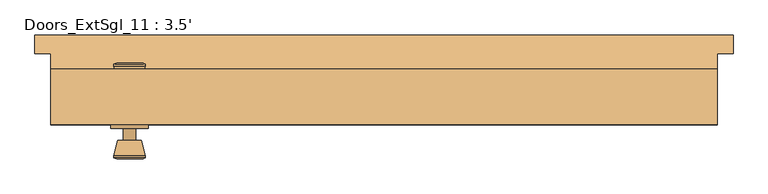
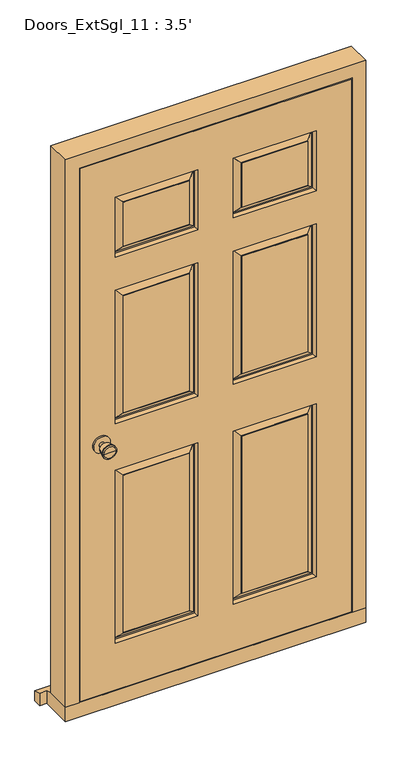
"""IFC4 building model written with IfcOpenShell, lengths in millimetres: door geometry, Doors_ExtSgl_11 : 3.5'."""

from ifc_helpers import new_model, si_unit, point, frame, frame_2d, origin, place, context, project, spatial, polyline, circle_curve, trimmed, segment, composite_curve, outline, extrude, faceted_brep, source, transform, mapped, element, save
from ifc_brep_helpers import plane_surface, cylinder_surface, revolved_surface, advanced_brep


def doors_extsgl_11_3_5_304e37c5(model_context):
    return source(origin(), model_context, "Body", "SolidModel", [
        advanced_brep(
        [(-406.9, 9.54, 1000.0), (-396.9, 9.54, 1000.0), (-416.9, 9.54, 1000.0), (-386.4241324, -39.46, 1000.0), (-406.9, -39.46, 1000.0), (-427.3758676, -39.46, 1000.0), (-381.9, -37.6321319, 1000.0), (-431.9, -37.6321319, 1000.0), (-381.9, -34.1684537, 1000.0), (-431.9, -34.1684537, 1000.0), (-388.263764, -9.46, 1000.0), (-425.536236, -9.46, 1000.0), (-396.9, -9.46, 1000.0), (-416.9, -9.46, 1000.0)],
        [
            (0, 1),
            (1, 2, circle_curve(frame((-406.9, 9.54, 1000.0), z_axis=(0.0, 1.0, 0.0), x_axis=(-1.0, 0.0, 0.0)), 10.0)),
            (2, 0),
            (2, 1, circle_curve(frame((-406.9, 9.54, 1000.0), z_axis=(0.0, 1.0, 0.0), x_axis=(-1.0, 0.0, 0.0)), 10.0)),
            (3, 4),
            (4, 5),
            (5, 3, circle_curve(frame((-406.9, -39.46, 1000.0), z_axis=(0.0, -1.0, 0.0), x_axis=(-1.0, 0.0, 0.0)), 20.4758676)),
            (3, 5, circle_curve(frame((-406.9, -39.46, 1000.0), z_axis=(0.0, -1.0, 0.0), x_axis=(-1.0, 0.0, 0.0)), 20.4758676)),
            (6, 3),
            (5, 7),
            (7, 6, circle_curve(frame((-406.9, -37.6321319, 1000.0), z_axis=(0.0, -1.0, 0.0), x_axis=(-1.0, 0.0, 0.0)), 25.0)),
            (6, 7, circle_curve(frame((-406.9, -37.6321319, 1000.0), z_axis=(0.0, -1.0, 0.0), x_axis=(-1.0, 0.0, 0.0)), 25.0)),
            (8, 6),
            (7, 9),
            (9, 8, circle_curve(frame((-406.9, -34.1684537, 1000.0), z_axis=(0.0, -1.0, 0.0), x_axis=(-1.0, 0.0, 0.0)), 25.0)),
            (8, 9, circle_curve(frame((-406.9, -34.1684537, 1000.0), z_axis=(0.0, -1.0, 0.0), x_axis=(-1.0, 0.0, 0.0)), 25.0)),
            (10, 8),
            (9, 11),
            (11, 10, circle_curve(frame((-406.9, -9.46, 1000.0), z_axis=(0.0, -1.0, 0.0), x_axis=(-1.0, 0.0, 0.0)), 18.636236)),
            (10, 11, circle_curve(frame((-406.9, -9.46, 1000.0), z_axis=(0.0, -1.0, 0.0), x_axis=(-1.0, 0.0, 0.0)), 18.636236)),
            (12, 10),
            (11, 13),
            (13, 12, circle_curve(frame((-406.9, -9.46, 1000.0), z_axis=(0.0, -1.0, 0.0), x_axis=(-1.0, 0.0, 0.0)), 10.0)),
            (12, 13, circle_curve(frame((-406.9, -9.46, 1000.0), z_axis=(0.0, -1.0, 0.0), x_axis=(-1.0, 0.0, 0.0)), 10.0)),
            (1, 12),
            (13, 2),
        ],
        [
            plane_surface(frame((-406.9, 9.54, 1000.0), z_axis=(0.0, 1.0, 0.0), x_axis=(-1.0, 0.0, 0.0))),
            plane_surface(frame((-406.9, -39.46, 1000.0), z_axis=(0.0, -1.0, 0.0), x_axis=(-1.0, 0.0, 0.0))),
            revolved_surface(polyline([(-427.3758676, -39.46, 1000.0), (-431.9, -37.6321319, 1000.0)]), (-406.9, 9.54, 1000.0), (0.0, 1.0, 0.0)),
            cylinder_surface(frame((-406.9, 9.54, 1000.0), z_axis=(0.0, 1.0, 0.0), x_axis=(-1.0, 0.0, 0.0)), 25.0),
            revolved_surface(polyline([(-431.9, -34.1684537, 1000.0), (-425.536236, -9.46, 1000.0)]), (-406.9, 9.54, 1000.0), (0.0, 1.0, 0.0)),
            plane_surface(frame((-406.9, -9.46, 1000.0), z_axis=(0.0, 1.0, 0.0), x_axis=(-1.0, 0.0, 0.0))),
            cylinder_surface(frame((-406.9, 9.54, 1000.0), z_axis=(0.0, 1.0, 0.0), x_axis=(-1.0, 0.0, 0.0)), 10.0),
        ],
        [
            (0, [[1, 2, 3]]),
            (0, [[-3, 4, -1]]),
            (1, [[5, 6, 7]]),
            (1, [[-6, -5, 8]]),
            (2, [[9, -7, 10, 11]]),
            (2, [[-10, -8, -9, 12]]),
            (3, [[13, -11, 14, 15]]),
            (3, [[-14, -12, -13, 16]]),
            (4, [[17, -15, 18, 19]]),
            (4, [[-18, -16, -17, 20]]),
            (5, [[21, -19, 22, 23]]),
            (5, [[-22, -20, -21, 24]]),
            (6, [[25, -23, 26, -2]]),
            (6, [[-26, -24, -25, -4]]),
        ],
    ),
        extrude(outline(composite_curve([segment(trimmed(circle_curve(frame_2d((1000.0, -406.9)), 30.0), [point((1000.0, -436.9))], [point((1000.0, -376.9))], False, "CARTESIAN"), True, "CONTINUOUS"), segment(trimmed(circle_curve(frame_2d((1000.0, -406.9)), 30.0), [point((1000.0, -376.9))], [point((1000.0, -436.9))], False, "CARTESIAN"), True, "CONTINUOUS")], self_intersect=False)), frame((0.0, 9.54, 0.0), z_axis=(0.0, 1.0, 0.0), x_axis=(0.0, 0.0, 1.0)), (0.0, 0.0, 1.0), 6.0),
        advanced_brep(
        [(-406.9, 65.54, 1000.0), (-416.9, 65.54, 1000.0), (-396.9, 65.54, 1000.0), (-386.4241324, 114.54, 1000.0), (-427.3758676, 114.54, 1000.0), (-406.9, 114.54, 1000.0), (-381.9, 112.7121319, 1000.0), (-431.9, 112.7121319, 1000.0), (-381.9, 109.2484537, 1000.0), (-431.9, 109.2484537, 1000.0), (-388.263764, 84.54, 1000.0), (-425.536236, 84.54, 1000.0), (-396.9, 84.54, 1000.0), (-416.9, 84.54, 1000.0)],
        [
            (0, 1),
            (1, 2, circle_curve(frame((-406.9, 65.54, 1000.0), z_axis=(0.0, -1.0, 0.0), x_axis=(-1.0, 0.0, 0.0)), 10.0)),
            (2, 0),
            (2, 1, circle_curve(frame((-406.9, 65.54, 1000.0), z_axis=(0.0, -1.0, 0.0), x_axis=(-1.0, 0.0, 0.0)), 10.0)),
            (3, 4, circle_curve(frame((-406.9, 114.54, 1000.0), z_axis=(0.0, 1.0, 0.0), x_axis=(-1.0, 0.0, 0.0)), 20.4758676)),
            (4, 5),
            (5, 3),
            (4, 3, circle_curve(frame((-406.9, 114.54, 1000.0), z_axis=(0.0, 1.0, 0.0), x_axis=(-1.0, 0.0, 0.0)), 20.4758676)),
            (6, 7, circle_curve(frame((-406.9, 112.7121319, 1000.0), z_axis=(0.0, 1.0, 0.0), x_axis=(-1.0, 0.0, 0.0)), 25.0)),
            (7, 4),
            (3, 6),
            (7, 6, circle_curve(frame((-406.9, 112.7121319, 1000.0), z_axis=(0.0, 1.0, 0.0), x_axis=(-1.0, 0.0, 0.0)), 25.0)),
            (8, 9, circle_curve(frame((-406.9, 109.2484537, 1000.0), z_axis=(0.0, 1.0, 0.0), x_axis=(-1.0, 0.0, 0.0)), 25.0)),
            (9, 7),
            (6, 8),
            (9, 8, circle_curve(frame((-406.9, 109.2484537, 1000.0), z_axis=(0.0, 1.0, 0.0), x_axis=(-1.0, 0.0, 0.0)), 25.0)),
            (10, 11, circle_curve(frame((-406.9, 84.54, 1000.0), z_axis=(0.0, 1.0, 0.0), x_axis=(-1.0, 0.0, 0.0)), 18.636236)),
            (11, 9),
            (8, 10),
            (11, 10, circle_curve(frame((-406.9, 84.54, 1000.0), z_axis=(0.0, 1.0, 0.0), x_axis=(-1.0, 0.0, 0.0)), 18.636236)),
            (12, 13, circle_curve(frame((-406.9, 84.54, 1000.0), z_axis=(0.0, 1.0, 0.0), x_axis=(-1.0, 0.0, 0.0)), 10.0)),
            (13, 11),
            (10, 12),
            (13, 12, circle_curve(frame((-406.9, 84.54, 1000.0), z_axis=(0.0, 1.0, 0.0), x_axis=(-1.0, 0.0, 0.0)), 10.0)),
            (1, 13),
            (12, 2),
        ],
        [
            plane_surface(frame((-406.9, 65.54, 1000.0), z_axis=(0.0, -1.0, 0.0), x_axis=(-1.0, 0.0, 0.0))),
            plane_surface(frame((-406.9, 114.54, 1000.0), z_axis=(0.0, 1.0, 0.0), x_axis=(-1.0, 0.0, 0.0))),
            revolved_surface(polyline([(-427.3758676, 114.54, 1000.0), (-431.9, 112.7121319, 1000.0)]), (-406.9, 65.54, 1000.0), (0.0, -1.0, 0.0)),
            cylinder_surface(frame((-406.9, 65.54, 1000.0), z_axis=(0.0, -1.0, 0.0), x_axis=(-1.0, 0.0, 0.0)), 25.0),
            revolved_surface(polyline([(-431.9, 109.2484537, 1000.0), (-425.536236, 84.54, 1000.0)]), (-406.9, 65.54, 1000.0), (0.0, -1.0, 0.0)),
            plane_surface(frame((-406.9, 84.54, 1000.0), z_axis=(0.0, -1.0, 0.0), x_axis=(-1.0, 0.0, 0.0))),
            cylinder_surface(frame((-406.9, 65.54, 1000.0), z_axis=(0.0, -1.0, 0.0), x_axis=(-1.0, 0.0, 0.0)), 10.0),
        ],
        [
            (0, [[1, 2, 3]]),
            (0, [[-3, 4, -1]]),
            (1, [[5, 6, 7]]),
            (1, [[8, -7, -6]]),
            (2, [[9, 10, -5, 11]]),
            (2, [[12, -11, -8, -10]]),
            (3, [[13, 14, -9, 15]]),
            (3, [[16, -15, -12, -14]]),
            (4, [[17, 18, -13, 19]]),
            (4, [[20, -19, -16, -18]]),
            (5, [[21, 22, -17, 23]]),
            (5, [[24, -23, -20, -22]]),
            (6, [[-2, 25, -21, 26]]),
            (6, [[-4, -26, -24, -25]]),
        ],
    ),
        extrude(outline(composite_curve([segment(trimmed(circle_curve(frame_2d((1000.0, -406.9)), 30.0), [point((1000.0, -436.9))], [point((1000.0, -376.9))], False, "CARTESIAN"), True, "CONTINUOUS"), segment(trimmed(circle_curve(frame_2d((1000.0, -406.9)), 30.0), [point((1000.0, -376.9))], [point((1000.0, -436.9))], False, "CARTESIAN"), True, "CONTINUOUS")], self_intersect=False)), frame((0.0, 59.54, 0.0), z_axis=(0.0, 1.0, 0.0), x_axis=(0.0, 0.0, 1.0)), (0.0, 0.0, 1.0), 6.0),
        faceted_brep([(462.9, 104.54, 54.5), (533.4, 104.54, 54.5), (533.4, 15.54, 54.5), (484.9, 15.54, 54.5), (484.9, 62.54, 54.5), (462.9, 62.54, 54.5), (462.9, 104.54, 2039.5), (-462.9, 104.54, 2039.5), (-462.9, 104.54, 54.5), (-533.4, 104.54, 54.5), (-533.4, 104.54, 2110.0), (533.4, 104.54, 2110.0), (533.4, 15.54, 2110.0), (-533.4, 15.54, 2110.0), (-533.4, 15.54, 54.5), (-484.9, 15.54, 54.5), (-484.9, 15.54, 2061.5), (484.9, 15.54, 2061.5), (484.9, 62.54, 2061.5), (-484.9, 62.54, 2061.5), (-484.9, 62.54, 54.5), (-462.9, 62.54, 54.5), (-462.9, 62.54, 2039.5), (462.9, 62.54, 2039.5)], [[[0, 1, 2, 3, 4, 5]], [[1, 0, 6, 7, 8, 9, 10, 11]], [[2, 1, 11, 12]], [[3, 2, 12, 13, 14, 15, 16, 17]], [[4, 3, 17, 18]], [[5, 4, 18, 19, 20, 21, 22, 23]], [[0, 5, 23, 6]], [[8, 7, 22, 21]], [[9, 8, 21, 20, 15, 14]], [[10, 9, 14, 13]], [[16, 15, 20, 19]], [[11, 10, 13, 12]], [[17, 16, 19, 18]], [[7, 6, 23, 22]]]),
        faceted_brep([(481.9, 15.54, 58.5), (481.9, 15.54, 2058.5), (-482.8250294, 15.54, 2058.5), (-482.8250294, 15.54, 58.5), (-62.5, 15.54, 883.5), (-62.5, 15.54, 233.5), (-356.9, 15.54, 233.5), (-356.9, 15.54, 883.5), (356.9, 15.54, 883.5), (356.9, 15.54, 233.5), (62.5, 15.54, 233.5), (62.5, 15.54, 883.5), (-62.5, 15.54, 1558.5), (-62.5, 15.54, 1058.5), (-356.9, 15.54, 1058.5), (-356.9, 15.54, 1558.5), (356.9, 15.54, 1558.5), (356.9, 15.54, 1058.5), (62.5, 15.54, 1058.5), (62.5, 15.54, 1558.5), (-62.5, 15.54, 1908.5), (-62.5, 15.54, 1683.5), (-356.9, 15.54, 1683.5), (-356.9, 15.54, 1908.5), (62.5, 15.54, 1683.5), (62.5, 15.54, 1908.5), (356.9, 15.54, 1908.5), (356.9, 15.54, 1683.5), (-92.5, 15.54, 263.5), (-92.5, 15.54, 853.5), (-326.9, 15.54, 853.5), (-326.9, 15.54, 263.5), (326.9, 15.54, 263.5), (326.9, 15.54, 853.5), (92.5, 15.54, 853.5), (92.5, 15.54, 263.5), (-92.5, 15.54, 1088.5), (-92.5, 15.54, 1528.5), (-326.9, 15.54, 1528.5), (-326.9, 15.54, 1088.5), (326.9, 15.54, 1088.5), (326.9, 15.54, 1528.5), (92.5, 15.54, 1528.5), (92.5, 15.54, 1088.5), (-92.5, 15.54, 1713.5), (-92.5, 15.54, 1878.5), (-326.9, 15.54, 1878.5), (-326.9, 15.54, 1713.5), (92.5, 15.54, 1878.5), (92.5, 15.54, 1713.5), (326.9, 15.54, 1713.5), (326.9, 15.54, 1878.5), (481.9, 59.54, 58.5), (-482.8250294, 59.54, 58.5), (-482.8250294, 59.54, 2058.5), (481.9, 59.54, 2058.5), (62.5, 59.54, 883.5), (62.5, 59.54, 233.5), (356.9, 59.54, 233.5), (356.9, 59.54, 883.5), (-356.9, 59.54, 883.5), (-356.9, 59.54, 233.5), (-62.5, 59.54, 233.5), (-62.5, 59.54, 883.5), (62.5, 59.54, 1558.5), (62.5, 59.54, 1058.5), (356.9, 59.54, 1058.5), (356.9, 59.54, 1558.5), (-356.9, 59.54, 1558.5), (-356.9, 59.54, 1058.5), (-62.5, 59.54, 1058.5), (-62.5, 59.54, 1558.5), (62.5, 59.54, 1908.5), (62.5, 59.54, 1683.5), (356.9, 59.54, 1683.5), (356.9, 59.54, 1908.5), (-356.9, 59.54, 1908.5), (-356.9, 59.54, 1683.5), (-62.5, 59.54, 1683.5), (-62.5, 59.54, 1908.5), (92.5, 59.54, 263.5), (92.5, 59.54, 853.5), (326.9, 59.54, 853.5), (326.9, 59.54, 263.5), (-326.9, 59.54, 263.5), (-326.9, 59.54, 853.5), (-92.5, 59.54, 853.5), (-92.5, 59.54, 263.5), (92.5, 59.54, 1088.5), (92.5, 59.54, 1528.5), (326.9, 59.54, 1528.5), (326.9, 59.54, 1088.5), (-326.9, 59.54, 1088.5), (-326.9, 59.54, 1528.5), (-92.5, 59.54, 1528.5), (-92.5, 59.54, 1088.5), (92.5, 59.54, 1713.5), (92.5, 59.54, 1878.5), (326.9, 59.54, 1878.5), (326.9, 59.54, 1713.5), (-326.9, 59.54, 1713.5), (-326.9, 59.54, 1878.5), (-92.5, 59.54, 1878.5), (-92.5, 59.54, 1713.5), (65.5, 44.54, 880.5), (65.5, 44.54, 236.5), (90.5, 58.54, 855.5), (90.5, 58.54, 261.5), (70.5, 44.54, 241.5), (70.5, 44.54, 875.5), (92.5, 58.54, 263.5), (92.5, 58.54, 853.5), (353.9, 44.54, 236.5), (328.9, 58.54, 261.5), (348.9, 44.54, 241.5), (326.9, 58.54, 263.5), (353.9, 44.54, 880.5), (328.9, 58.54, 855.5), (348.9, 44.54, 875.5), (326.9, 58.54, 853.5), (-353.9, 44.54, 880.5), (-353.9, 44.54, 236.5), (-328.9, 58.54, 855.5), (-328.9, 58.54, 261.5), (-348.9, 44.54, 241.5), (-348.9, 44.54, 875.5), (-326.9, 58.54, 263.5), (-326.9, 58.54, 853.5), (-65.5, 44.54, 236.5), (-90.5, 58.54, 261.5), (-70.5, 44.54, 241.5), (-92.5, 58.54, 263.5), (-65.5, 44.54, 880.5), (-90.5, 58.54, 855.5), (-70.5, 44.54, 875.5), (-92.5, 58.54, 853.5), (-92.5, 16.54, 263.5), (-92.5, 16.54, 853.5), (-70.5, 30.54, 241.5), (-70.5, 30.54, 875.5), (-90.5, 16.54, 855.5), (-90.5, 16.54, 261.5), (-65.5, 30.54, 880.5), (-65.5, 30.54, 236.5), (-326.9, 16.54, 853.5), (-348.9, 30.54, 875.5), (-328.9, 16.54, 855.5), (-353.9, 30.54, 880.5), (-326.9, 16.54, 263.5), (-348.9, 30.54, 241.5), (-328.9, 16.54, 261.5), (-353.9, 30.54, 236.5), (353.9, 30.54, 880.5), (353.9, 30.54, 236.5), (328.9, 16.54, 855.5), (328.9, 16.54, 261.5), (348.9, 30.54, 241.5), (348.9, 30.54, 875.5), (326.9, 16.54, 263.5), (326.9, 16.54, 853.5), (65.5, 30.54, 236.5), (90.5, 16.54, 261.5), (70.5, 30.54, 241.5), (92.5, 16.54, 263.5), (65.5, 30.54, 880.5), (90.5, 16.54, 855.5), (70.5, 30.54, 875.5), (92.5, 16.54, 853.5), (92.5, 58.54, 1088.5), (92.5, 58.54, 1528.5), (70.5, 44.54, 1066.5), (70.5, 44.54, 1550.5), (90.5, 58.54, 1530.5), (90.5, 58.54, 1086.5), (65.5, 44.54, 1555.5), (65.5, 44.54, 1061.5), (326.9, 58.54, 1528.5), (348.9, 44.54, 1550.5), (328.9, 58.54, 1530.5), (353.9, 44.54, 1555.5), (326.9, 58.54, 1088.5), (348.9, 44.54, 1066.5), (328.9, 58.54, 1086.5), (353.9, 44.54, 1061.5), (-326.9, 58.54, 1088.5), (-326.9, 58.54, 1528.5), (-348.9, 44.54, 1066.5), (-348.9, 44.54, 1550.5), (-328.9, 58.54, 1530.5), (-328.9, 58.54, 1086.5), (-353.9, 44.54, 1555.5), (-353.9, 44.54, 1061.5), (-92.5, 58.54, 1528.5), (-70.5, 44.54, 1550.5), (-90.5, 58.54, 1530.5), (-65.5, 44.54, 1555.5), (-92.5, 58.54, 1088.5), (-70.5, 44.54, 1066.5), (-90.5, 58.54, 1086.5), (-65.5, 44.54, 1061.5), (-92.5, 16.54, 1088.5), (-92.5, 16.54, 1528.5), (-70.5, 30.54, 1066.5), (-70.5, 30.54, 1550.5), (-90.5, 16.54, 1530.5), (-90.5, 16.54, 1086.5), (-65.5, 30.54, 1555.5), (-65.5, 30.54, 1061.5), (-326.9, 16.54, 1528.5), (-348.9, 30.54, 1550.5), (-328.9, 16.54, 1530.5), (-353.9, 30.54, 1555.5), (-326.9, 16.54, 1088.5), (-348.9, 30.54, 1066.5), (-328.9, 16.54, 1086.5), (-353.9, 30.54, 1061.5), (353.9, 30.54, 1555.5), (353.9, 30.54, 1061.5), (328.9, 16.54, 1530.5), (328.9, 16.54, 1086.5), (348.9, 30.54, 1066.5), (348.9, 30.54, 1550.5), (326.9, 16.54, 1088.5), (326.9, 16.54, 1528.5), (65.5, 30.54, 1061.5), (90.5, 16.54, 1086.5), (70.5, 30.54, 1066.5), (92.5, 16.54, 1088.5), (65.5, 30.54, 1555.5), (90.5, 16.54, 1530.5), (70.5, 30.54, 1550.5), (92.5, 16.54, 1528.5), (92.5, 58.54, 1713.5), (92.5, 58.54, 1878.5), (70.5, 44.54, 1691.5), (70.5, 44.54, 1900.5), (90.5, 58.54, 1880.5), (90.5, 58.54, 1711.5), (65.5, 44.54, 1905.5), (65.5, 44.54, 1686.5), (326.9, 58.54, 1878.5), (348.9, 44.54, 1900.5), (328.9, 58.54, 1880.5), (353.9, 44.54, 1905.5), (326.9, 58.54, 1713.5), (348.9, 44.54, 1691.5), (328.9, 58.54, 1711.5), (353.9, 44.54, 1686.5), (-326.9, 58.54, 1713.5), (-326.9, 58.54, 1878.5), (-348.9, 44.54, 1691.5), (-348.9, 44.54, 1900.5), (-328.9, 58.54, 1880.5), (-328.9, 58.54, 1711.5), (-353.9, 44.54, 1905.5), (-353.9, 44.54, 1686.5), (-92.5, 58.54, 1878.5), (-70.5, 44.54, 1900.5), (-90.5, 58.54, 1880.5), (-65.5, 44.54, 1905.5), (-92.5, 58.54, 1713.5), (-70.5, 44.54, 1691.5), (-90.5, 58.54, 1711.5), (-65.5, 44.54, 1686.5), (-92.5, 16.54, 1713.5), (-92.5, 16.54, 1878.5), (-70.5, 30.54, 1691.5), (-70.5, 30.54, 1900.5), (-90.5, 16.54, 1880.5), (-90.5, 16.54, 1711.5), (-65.5, 30.54, 1905.5), (-65.5, 30.54, 1686.5), (-326.9, 16.54, 1878.5), (-348.9, 30.54, 1900.5), (-328.9, 16.54, 1880.5), (-353.9, 30.54, 1905.5), (-326.9, 16.54, 1713.5), (-348.9, 30.54, 1691.5), (-328.9, 16.54, 1711.5), (-353.9, 30.54, 1686.5), (92.5, 16.54, 1878.5), (92.5, 16.54, 1713.5), (70.5, 30.54, 1900.5), (70.5, 30.54, 1691.5), (90.5, 16.54, 1711.5), (90.5, 16.54, 1880.5), (65.5, 30.54, 1686.5), (65.5, 30.54, 1905.5), (326.9, 16.54, 1713.5), (348.9, 30.54, 1691.5), (328.9, 16.54, 1711.5), (353.9, 30.54, 1686.5), (326.9, 16.54, 1878.5), (348.9, 30.54, 1900.5), (328.9, 16.54, 1880.5), (353.9, 30.54, 1905.5)], [[[0, 1, 2, 3], [4, 5, 6, 7], [8, 9, 10, 11], [12, 13, 14, 15], [16, 17, 18, 19], [20, 21, 22, 23], [24, 25, 26, 27]], [[28, 29, 30, 31]], [[32, 33, 34, 35]], [[36, 37, 38, 39]], [[40, 41, 42, 43]], [[44, 45, 46, 47]], [[48, 49, 50, 51]], [[52, 53, 54, 55], [56, 57, 58, 59], [60, 61, 62, 63], [64, 65, 66, 67], [68, 69, 70, 71], [72, 73, 74, 75], [76, 77, 78, 79]], [[80, 81, 82, 83]], [[84, 85, 86, 87]], [[88, 89, 90, 91]], [[92, 93, 94, 95]], [[96, 97, 98, 99]], [[100, 101, 102, 103]], [[1, 0, 52, 55]], [[2, 1, 55, 54]], [[3, 2, 54, 53]], [[0, 3, 53, 52]], [[104, 105, 57, 56]], [[106, 107, 108, 109]], [[80, 110, 111, 81]], [[57, 105, 112, 58]], [[108, 107, 113, 114]], [[110, 80, 83, 115]], [[58, 112, 116, 59]], [[114, 113, 117, 118]], [[115, 83, 82, 119]], [[104, 56, 59, 116]], [[105, 104, 116, 112], [109, 108, 114, 118]], [[106, 109, 118, 117]], [[107, 106, 117, 113], [111, 110, 115, 119]], [[81, 111, 119, 82]], [[120, 121, 61, 60]], [[122, 123, 124, 125]], [[84, 126, 127, 85]], [[61, 121, 128, 62]], [[124, 123, 129, 130]], [[126, 84, 87, 131]], [[62, 128, 132, 63]], [[130, 129, 133, 134]], [[131, 87, 86, 135]], [[120, 60, 63, 132]], [[121, 120, 132, 128], [125, 124, 130, 134]], [[122, 125, 134, 133]], [[123, 122, 133, 129], [127, 126, 131, 135]], [[85, 127, 135, 86]], [[136, 137, 29, 28]], [[138, 139, 140, 141]], [[4, 142, 143, 5]], [[29, 137, 144, 30]], [[140, 139, 145, 146]], [[142, 4, 7, 147]], [[30, 144, 148, 31]], [[146, 145, 149, 150]], [[147, 7, 6, 151]], [[136, 28, 31, 148]], [[141, 140, 146, 150], [137, 136, 148, 144]], [[138, 141, 150, 149]], [[143, 142, 147, 151], [139, 138, 149, 145]], [[5, 143, 151, 6]], [[152, 153, 9, 8]], [[154, 155, 156, 157]], [[32, 158, 159, 33]], [[9, 153, 160, 10]], [[156, 155, 161, 162]], [[158, 32, 35, 163]], [[10, 160, 164, 11]], [[162, 161, 165, 166]], [[163, 35, 34, 167]], [[152, 8, 11, 164]], [[153, 152, 164, 160], [157, 156, 162, 166]], [[154, 157, 166, 165]], [[155, 154, 165, 161], [159, 158, 163, 167]], [[33, 159, 167, 34]], [[168, 169, 89, 88]], [[170, 171, 172, 173]], [[64, 174, 175, 65]], [[89, 169, 176, 90]], [[172, 171, 177, 178]], [[174, 64, 67, 179]], [[90, 176, 180, 91]], [[178, 177, 181, 182]], [[179, 67, 66, 183]], [[168, 88, 91, 180]], [[173, 172, 178, 182], [169, 168, 180, 176]], [[170, 173, 182, 181]], [[175, 174, 179, 183], [171, 170, 181, 177]], [[65, 175, 183, 66]], [[184, 185, 93, 92]], [[186, 187, 188, 189]], [[68, 190, 191, 69]], [[93, 185, 192, 94]], [[188, 187, 193, 194]], [[190, 68, 71, 195]], [[94, 192, 196, 95]], [[194, 193, 197, 198]], [[195, 71, 70, 199]], [[184, 92, 95, 196]], [[189, 188, 194, 198], [185, 184, 196, 192]], [[186, 189, 198, 197]], [[191, 190, 195, 199], [187, 186, 197, 193]], [[69, 191, 199, 70]], [[200, 201, 37, 36]], [[202, 203, 204, 205]], [[12, 206, 207, 13]], [[37, 201, 208, 38]], [[204, 203, 209, 210]], [[206, 12, 15, 211]], [[38, 208, 212, 39]], [[210, 209, 213, 214]], [[211, 15, 14, 215]], [[200, 36, 39, 212]], [[205, 204, 210, 214], [201, 200, 212, 208]], [[202, 205, 214, 213]], [[207, 206, 211, 215], [203, 202, 213, 209]], [[13, 207, 215, 14]], [[216, 217, 17, 16]], [[218, 219, 220, 221]], [[40, 222, 223, 41]], [[17, 217, 224, 18]], [[220, 219, 225, 226]], [[222, 40, 43, 227]], [[18, 224, 228, 19]], [[226, 225, 229, 230]], [[227, 43, 42, 231]], [[216, 16, 19, 228]], [[217, 216, 228, 224], [221, 220, 226, 230]], [[218, 221, 230, 229]], [[219, 218, 229, 225], [223, 222, 227, 231]], [[41, 223, 231, 42]], [[232, 233, 97, 96]], [[234, 235, 236, 237]], [[72, 238, 239, 73]], [[97, 233, 240, 98]], [[236, 235, 241, 242]], [[238, 72, 75, 243]], [[98, 240, 244, 99]], [[242, 241, 245, 246]], [[243, 75, 74, 247]], [[232, 96, 99, 244]], [[237, 236, 242, 246], [233, 232, 244, 240]], [[234, 237, 246, 245]], [[239, 238, 243, 247], [235, 234, 245, 241]], [[73, 239, 247, 74]], [[248, 249, 101, 100]], [[250, 251, 252, 253]], [[76, 254, 255, 77]], [[101, 249, 256, 102]], [[252, 251, 257, 258]], [[254, 76, 79, 259]], [[102, 256, 260, 103]], [[258, 257, 261, 262]], [[259, 79, 78, 263]], [[248, 100, 103, 260]], [[253, 252, 258, 262], [249, 248, 260, 256]], [[250, 253, 262, 261]], [[255, 254, 259, 263], [251, 250, 261, 257]], [[77, 255, 263, 78]], [[264, 265, 45, 44]], [[266, 267, 268, 269]], [[20, 270, 271, 21]], [[45, 265, 272, 46]], [[268, 267, 273, 274]], [[270, 20, 23, 275]], [[46, 272, 276, 47]], [[274, 273, 277, 278]], [[275, 23, 22, 279]], [[264, 44, 47, 276]], [[269, 268, 274, 278], [265, 264, 276, 272]], [[266, 269, 278, 277]], [[271, 270, 275, 279], [267, 266, 277, 273]], [[21, 271, 279, 22]], [[280, 281, 49, 48]], [[282, 283, 284, 285]], [[24, 286, 287, 25]], [[49, 281, 288, 50]], [[284, 283, 289, 290]], [[286, 24, 27, 291]], [[50, 288, 292, 51]], [[290, 289, 293, 294]], [[291, 27, 26, 295]], [[280, 48, 51, 292]], [[285, 284, 290, 294], [281, 280, 292, 288]], [[282, 285, 294, 293]], [[287, 286, 291, 295], [283, 282, 293, 289]], [[25, 287, 295, 26]]]),
        faceted_brep([(558.4, 159.54, 0.0), (558.4, 159.54, 38.5947221), (558.4, 129.54, 47.2703282), (558.4, 129.54, 0.0), (-558.4, 159.54, 38.5947221), (-558.4, 159.54, 0.0), (-558.4, 129.54, 0.0), (-558.4, 129.54, 47.2703282), (533.4, 129.54, 0.0), (533.4, 15.54, 0.0), (-533.4, 15.54, 0.0), (-533.4, 129.54, 0.0), (-533.4, 129.54, 47.2703282), (-533.4, 104.54, 54.5), (533.4, 104.54, 54.5), (533.4, 129.54, 47.2703282), (-533.4, 15.54, 54.5), (533.4, 15.54, 54.5)], [[[0, 1, 2, 3]], [[4, 5, 6, 7]], [[5, 0, 3, 8, 9, 10, 11, 6]], [[1, 0, 5, 4]], [[1, 4, 7, 12, 13, 14, 15, 2]], [[13, 16, 17, 14]], [[16, 10, 9, 17]], [[12, 11, 10, 16, 13]], [[11, 12, 7, 6]], [[8, 15, 14, 17, 9]], [[15, 8, 3, 2]]]),
    ])


if __name__ == "__main__":
    model = new_model("IFC4")
    model_context = context("Model", 3, world=origin())
    ifc_project = project(units=[si_unit("LENGTHUNIT", "METRE", prefix="MILLI")], contexts=[model_context])
    site = spatial("IfcSite", under=ifc_project)
    building = spatial("IfcBuilding", under=site)
    placement = place(None, origin())
    doors_extsgl_11_3_5_shape = doors_extsgl_11_3_5_304e37c5(model_context)
    element("IfcDoor", 1, ObjectType="Doors_ExtSgl_11 : 3.5'", at=placement, inside=building, context=model_context, shape_type="MappedRepresentation", body=[
        mapped(doors_extsgl_11_3_5_shape, transform((0.0, 0.0, 0.0), x_axis=(1.0, 0.0, 0.0), y_axis=(0.0, 1.0, 0.0), z_axis=(0.0, 0.0, 1.0))),
    ])
    save(model, "model.ifc")

# Revit data of these elements
# Type "Doors_ExtSgl_11 : 3.5'"
#   Type Mark = "48"
#   Type Comments = "External Single"
#   Operation = "SingleSwingRight"
#   Construction Type Id = "MDOOR"
#   Keynote = "L20"
#   Analytic Construction = "Metal"
#   Wrap Layers (Int) from Ext = 177.5 mm
#   Wrap Layers (Ext) from Ext = 102.5 mm
#   Thickness = 44 mm
#   Stile Top of Lock rail = 1000 mm
#   Stile Top of Frieze Rail = 1625 mm
#   Stile Top Rail = 150 mm
#   Stile Shutting = 125 mm
#   Stile Muntin Rail = 125 mm
#   Stile Lock Rail = 175 mm
#   Stile Intermediate/Frieze = 125 mm
#   Stile Hanging = 125 mm
#   Stile Bottom Rail = 175 mm
#   Rough Width = 1066.8 mm
#   Rough Height = 2110 mm
#   O/A Frame Width = 64 mm
#   Heat Transfer Coefficient (U) = 3.7021 W/(m²·K)
#   Handle Z Distance = 1000 mm
#   Glazing Thickness = 24 mm
#   FrameWidth = 42 mm
#   FrameOffset - External = 25 mm
#   FrameDepth = 89 mm
#   Door Panel Width = 963.8 mm
#   Door Panel Thickness = 44 mm
#   Door Panel Height = 2000 mm
#   Cill Thickness = 54.5 mm
#   Handle X Distance = 75 mm
#   Height = 2110 mm
#   Structural Tolerance = 6.5 mm
#   Tolerance = 3 mm
#   Undercut = 4 mm
#   Width = 1066.8 mm
#   Cill Projection = 30 mm
#   Cill Extension = 25 mm
#   Cavity Closer Width = 50 mm
#   Cavity Closer Offset from Ext = 102.5 mm
#   Cavity Closer Depth = 85 mm
#   Vis - Ironmongery = yes
#   Vis - Cavity Closers = yes
#   Define Thermal Properties by = 1
#   Function = 1
#   Material Door = Door - Panel
#   Material Frame = Door - Frame/Mullion
#   Material Ironmongery = Door - Handle
#   Visual Light Transmittance = 0
#   Solar Heat Gain Coefficient = 0
#   Wall Closure = (empty or 0)
# Element 1 (IfcDoor, "Doors_ExtSgl_11 : 3.5'")
#   Materials on its faces: "Door - Panel", "Door - Handle", "Door - Frame/Mullion"
# Materials
#   "Door - Panel": class "Wood", colour RGB 210 159 95, transparency 0, Keynote = "L20", Cost = 0
#   "Door - Frame/Mullion": class "Wood", colour RGB 212 179 113, transparency 0, Keynote = "L20", Cost = 0
#   "Door - Handle": colour RGB 0 0 0, transparency 0, Keynote = "P21", Cost = 0
